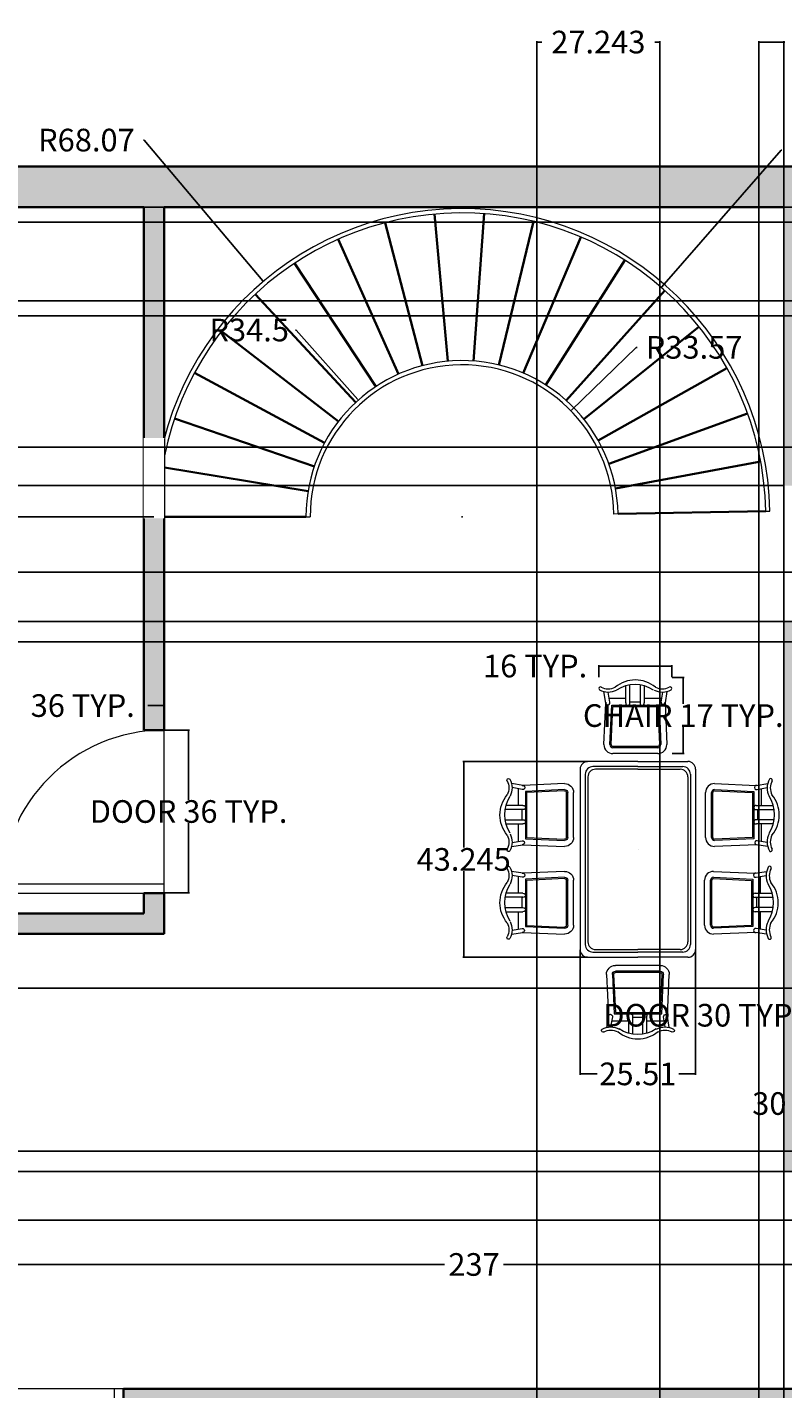
# Model space of a CAD drawing. Units: inches. Extents: x 2807 to 3326, y 2005 to 2580.
# Tile 10 of 12: x 2968 to 3135, y 2280 to 2580. Entities that reach past the tile are written whole.
import ezdxf

# ---------------------------------------------------------------- set-up
doc = ezdxf.new("R2010")
doc.units = ezdxf.units.IN
doc.header["$LTSCALE"] = 0.4
doc.set_wipeout_variables(frame=1)
for name, color, linetype, lineweight in [('A-ANNO-DIMS', 2, 'Continuous', 18), ('A-FLOR-STRS', 233, 'Continuous', 18), ('A-WALL-PATT', 231, 'Continuous', 13), ('DOORS', 144, 'Continuous', 18), ('Furniture', 7, 'Continuous', 15), ('WALL', 233, 'Continuous', 35)]:
    doc.layers.add(name, color=color, linetype=linetype, lineweight=lineweight)
doc.styles.get("Standard").update_dxf_attribs({"font": 'txt', "height": 5})
doc.dimstyles.get("Standard").update_dxf_attribs({"dimtxt": 0.18, "dimasz": 0.18, "dimexe": 0.18, "dimexo": 0.0625, "dimgap": 0.09, "dimtad": 0, "dimtih": 1, "dimtoh": 1, "dimdec": 4, "dimzin": 0, "dimdsep": 46, "dimtxsty": 'Standard', "dimcen": 0.09, "dimadec": 0, "dimazin": 0, "dimtfac": 1, "dimtdec": 4, "dimtofl": 0, "dimtmove": 0, "dimatfit": 3, "dimfxl": 1, "dimtolj": 1, "dimtzin": 0, "dimarcsym": 0})

# ---------------------------------------------------------------- blocks, each defined once
blk = doc.blocks.new('*U1')
at = {"layer": 'WALL'}
blk.add_line((0, -0.93), (0, -33.57), dxfattribs=at)
blk = doc.blocks.new('*U2')
at = {"layer": 'A-FLOR-STRS', "transparency": 16777216}
for p, rotation in [((3057.71, 2539.95), 5.233641268316883), ((3068.89, 2540.06), 355.8151569647967), ((3046.7, 2538.02), 14.65212557183719), ((3079.93, 2538.33), 346.3966726612762), ((3036.16, 2534.32), 24.07060987535752), ((3090.54, 2534.82), 336.9781883577561), ((3026.36, 2528.94), 33.48909417887789), ((3100.43, 2529.62), 327.5597040542357), ((3017.58, 2522.03), 42.90757848239826), ((3109.34, 2522.87), 318.1412197507153), ((3117.02, 2514.75), 308.7227354471949), ((3010.04, 2513.77), 52.32606278591863), ((3003.96, 2504.39), 61.74454708943897), ((3123.28, 2505.49), 299.3042511436746), ((2999.5, 2494.15), 71.16303139295928), ((3127.93, 2495.32), 289.8857668401543), ((3130.85, 2484.54), 280.4672825366339), ((2996.77, 2483.31), 80.58151569647963), ((2995.85, 2472.17), 90), ((3131.98, 2473.42), 271.0487982331135)]:
    blk.add_blockref('*U1', p, dxfattribs=dict(at, rotation=rotation))
blk = doc.blocks.new('DOOR-36')
for p, q in [((0, 0), (-36, 0)), ((-2, -35.94), (-2, 0)), ((0, -36), (0, 0))]:
    blk.add_line(p, q)
blk.add_arc((0, 0), 36, 180, 270)
blk = doc.blocks.new('CHAIR-DINING')
for p, q in [((-6.16, 6.94), (3.02, 6.53)), ((3.02, 6.53), (5.58, 6.94)), ((3.24, 5.62), (5.46, 6.04)), ((-8.14, -4.96), (-8.14, 4.96)), ((-6.84, -4.96), (-6.84, 4.96)), ((-6.56, -4.96), (-6.56, 4.96)), ((-6.16, 5.36), (2.25, 4.95)), ((-6.15, 5.64), (2.53, 5.22)), ((2.25, 4.95), (2.25, -5)), ((2.53, 5.22), (2.53, -5.28)), ((4.12, 5.78), (4.12, 2.1)), ((3.07, 2.1), (6.82, 2.1)), ((3.07, 1.2), (7.01, 1.2)), ((3.32, 1.2), (3.32, -1.08)), ((7.02, -1.08), (3.07, -1.08)), ((6.82, -1.98), (3.08, -1.98)), ((4.12, -1.98), (4.12, -5.82)), ((2.25, -5), (-6.16, -5.36)), ((2.53, -5.28), (-6.15, -5.64)), ((5.46, -6.04), (3.24, -5.67)), ((3.1, -6.58), (-6.16, -6.95)), ((5.58, -6.95), (3.1, -6.58))]:
    blk.add_line(p, q)
for centre, radius, start, end in [((-6.16, 4.96), 1.98, 90, 180), ((3.13, 6.07), 0.467, 76.2748, 283.7252), ((9.44, 5.97), 3.98, 151.1173, 207.5141), ((6.25, 7.7), 0.355, 326.5726, 147.7215), ((9.44, 5.97), 3.28, 150.9211, 207.5141), ((-6.16, 4.96), 0.68, 90, 180), ((-6.16, 4.96), 0.397, 90, 180), ((-0.48, 0.05), 7.58, 327.3186, 32.6814), ((1.16, 0), 6.98, 320.3459, 39.6541), ((2.98, 1.65), 0.463, 78.6748, 281.3252), ((2.98, -1.53), 0.463, 78.8014, 282.2085), ((-6.16, -4.96), 1.98, 180, 270), ((-6.16, -4.96), 0.68, 180, 270), ((-6.16, -4.96), 0.397, 180, 270), ((3.17, -6.13), 0.459, 80.8614, 279.1386), ((9.44, -5.97), 3.98, 152.4859, 208.8827), ((9.44, -5.97), 3.28, 152.4859, 208.022), ((6.25, -7.71), 0.355, 212.2785, 33.4274)]:
    blk.add_arc(centre, radius, start, end)
blk = doc.blocks.new('*D17')
at = {"layer": 'A-ANNO-DIMS', "color": 0, "lineweight": -2, "ltscale": 0.4, "transparency": 16777216}
for p, q in [((2998.13, 2425.08), (3003.65, 2425.08)), ((3003.47, 2424.9), (3003.47, 2409.67)), ((3003.47, 2389.26), (3003.47, 2404.49)), ((2998.13, 2389.08), (3003.65, 2389.08))]:
    blk.add_line(p, q, dxfattribs=at)
at = {"layer": 'A-ANNO-DIMS', "color": 0, "ltscale": 0.4, "transparency": 16777216}
for points in [[(3003.44, 2424.9), (3003.5, 2424.9), (3003.47, 2425.08)], [(3003.44, 2389.26), (3003.5, 2389.26), (3003.47, 2389.08)]]:
    blk.add_solid(points, dxfattribs=at)
at = {"layer": 'Defpoints', "color": 0, "ltscale": 0.4, "transparency": 16777216}
for p in [(2998.07, 2425.08), (2998.07, 2389.08), (3003.47, 2389.08)]:
    blk.add_point(p, dxfattribs=at)
at = {"layer": 'A-ANNO-DIMS', "color": 0, "ltscale": 0.4, "transparency": 16777216, "insert": (3003.47, 2407.08), "char_height": 5, "attachment_point": 5}
blk.add_mtext('\\A1;DOOR 36 TYP.', dxfattribs=at)
blk = doc.blocks.new('*D18')
at = {"layer": 'A-ANNO-DIMS', "color": 0, "lineweight": -2, "ltscale": 0.4, "transparency": 16777216}
for p, q in [((2962.07, 2425.14), (2962.07, 2430.66)), ((2962.25, 2430.48), (2965.69, 2430.48)), ((2997.89, 2430.48), (2994.44, 2430.48)), ((2998.07, 2425.14), (2998.07, 2430.66))]:
    blk.add_line(p, q, dxfattribs=at)
at = {"layer": 'A-ANNO-DIMS', "color": 0, "ltscale": 0.4, "transparency": 16777216}
for points in [[(2962.25, 2430.51), (2962.25, 2430.45), (2962.07, 2430.48)], [(2997.89, 2430.51), (2997.89, 2430.45), (2998.07, 2430.48)]]:
    blk.add_solid(points, dxfattribs=at)
at = {"layer": 'Defpoints', "color": 0, "ltscale": 0.4, "transparency": 16777216}
for p in [(2998.07, 2430.48), (2962.07, 2425.08), (2998.07, 2425.08)]:
    blk.add_point(p, dxfattribs=at)
at = {"layer": 'A-ANNO-DIMS', "color": 0, "ltscale": 0.4, "transparency": 16777216, "insert": (2980.07, 2430.48), "char_height": 5, "attachment_point": 5}
blk.add_mtext('\\A1;36 TYP.', dxfattribs=at)
blk = doc.blocks.new('*D19')
at = {"layer": 'A-ANNO-DIMS', "color": 0, "lineweight": -2, "ltscale": 0.4, "transparency": 16777216}
for p, q in [((3144.07, 2362.08), (3143.89, 2362.08)), ((3144.07, 2357.64), (3144.07, 2362.26)), ((3173.89, 2362.08), (3144.25, 2362.08)), ((3174.07, 2357.64), (3174.07, 2362.26))]:
    blk.add_line(p, q, dxfattribs=at)
at = {"layer": 'A-ANNO-DIMS', "color": 0, "ltscale": 0.4, "transparency": 16777216}
for points in [[(3144.25, 2362.11), (3144.25, 2362.05), (3144.07, 2362.08)], [(3173.89, 2362.11), (3173.89, 2362.05), (3174.07, 2362.08)]]:
    blk.add_solid(points, dxfattribs=at)
at = {"layer": 'Defpoints', "color": 0, "ltscale": 0.4, "transparency": 16777216}
for p in [(3144.07, 2362.08), (3144.07, 2357.58), (3174.07, 2357.58)]:
    blk.add_point(p, dxfattribs=at)
at = {"layer": 'A-ANNO-DIMS', "color": 0, "ltscale": 0.4, "transparency": 16777216, "insert": (3117.01, 2362.08), "char_height": 5, "attachment_point": 5}
blk.add_mtext('\\A1;DOOR 30 TYP.', dxfattribs=at)
blk = doc.blocks.new('*D20')
at = {"layer": 'A-ANNO-DIMS', "color": 0, "lineweight": -2, "ltscale": 0.4, "transparency": 16777216}
for p, q in [((3144, 2357.58), (3139.39, 2357.58)), ((3139.57, 2357.4), (3139.57, 2345.17)), ((3139.57, 2327.76), (3139.57, 2339.99)), ((3144, 2327.58), (3139.39, 2327.58))]:
    blk.add_line(p, q, dxfattribs=at)
at = {"layer": 'A-ANNO-DIMS', "color": 0, "ltscale": 0.4, "transparency": 16777216}
for points in [[(3139.54, 2357.4), (3139.6, 2357.4), (3139.57, 2357.58)], [(3139.54, 2327.76), (3139.6, 2327.76), (3139.57, 2327.58)]]:
    blk.add_solid(points, dxfattribs=at)
at = {"layer": 'Defpoints', "color": 0, "ltscale": 0.4, "transparency": 16777216}
for p in [(3144.07, 2357.58), (3139.57, 2327.58), (3144.07, 2327.58)]:
    blk.add_point(p, dxfattribs=at)
at = {"layer": 'A-ANNO-DIMS', "color": 0, "ltscale": 0.4, "transparency": 16777216, "insert": (3139.57, 2342.58), "char_height": 5, "attachment_point": 5}
blk.add_mtext('\\A1;30 TYP.', dxfattribs=at)
blk = doc.blocks.new('*D27')
at = {"layer": 'A-ANNO-DIMS', "color": 0, "lineweight": -2, "ltscale": 0.4, "transparency": 16777216}
for p, q in [((3110.36, 2436.69), (3113, 2436.69)), ((3112.82, 2436.51), (3112.82, 2430.86)), ((3112.82, 2420.04), (3112.82, 2425.68)), ((3110.36, 2419.86), (3113, 2419.86))]:
    blk.add_line(p, q, dxfattribs=at)
at = {"layer": 'A-ANNO-DIMS', "color": 0, "ltscale": 0.4, "transparency": 16777216}
for points in [[(3112.79, 2436.51), (3112.85, 2436.51), (3112.82, 2436.69)], [(3112.79, 2420.04), (3112.85, 2420.04), (3112.82, 2419.86)]]:
    blk.add_solid(points, dxfattribs=at)
at = {"layer": 'Defpoints', "color": 0, "ltscale": 0.4, "transparency": 16777216}
for p in [(3110.29, 2436.69), (3112.82, 2436.69), (3110.29, 2419.86)]:
    blk.add_point(p, dxfattribs=at)
at = {"layer": 'A-ANNO-DIMS', "color": 0, "ltscale": 0.4, "transparency": 16777216, "insert": (3112.82, 2428.27), "char_height": 5, "attachment_point": 5}
blk.add_mtext('\\A1;CHAIR 17 TYP.', dxfattribs=at)
blk = doc.blocks.new('*D28')
at = {"layer": 'A-ANNO-DIMS', "color": 0, "lineweight": -2, "ltscale": 0.4, "transparency": 16777216}
for p, q in [((3094.16, 2439.21), (3093.98, 2439.21)), ((3094.16, 2436.75), (3094.16, 2439.39)), ((3110.11, 2439.21), (3094.34, 2439.21)), ((3110.29, 2436.75), (3110.29, 2439.39))]:
    blk.add_line(p, q, dxfattribs=at)
at = {"layer": 'A-ANNO-DIMS', "color": 0, "ltscale": 0.4, "transparency": 16777216}
for points in [[(3094.34, 2439.24), (3094.34, 2439.18), (3094.16, 2439.21)], [(3110.11, 2439.24), (3110.11, 2439.18), (3110.29, 2439.21)]]:
    blk.add_solid(points, dxfattribs=at)
at = {"layer": 'Defpoints', "color": 0, "ltscale": 0.4, "transparency": 16777216}
for p in [(3094.16, 2439.21), (3094.16, 2436.69), (3110.29, 2436.69)]:
    blk.add_point(p, dxfattribs=at)
at = {"layer": 'A-ANNO-DIMS', "color": 0, "ltscale": 0.4, "transparency": 16777216, "insert": (3080.08, 2439.21), "char_height": 5, "attachment_point": 5}
blk.add_mtext('\\A1;16 TYP.', dxfattribs=at)
blk = doc.blocks.new('*D46')
at = {"layer": 'A-ANNO-DIMS', "color": 0, "lineweight": -2, "ltscale": 0.4, "transparency": 16777216}
for p, q in [((3279.5, 2327.58), (2816.94, 2327.58)), ((2817.12, 2327.4), (2817.12, 2324.79)), ((2817.12, 2317), (2817.12, 2319.61)), ((3279.5, 2316.82), (2816.94, 2316.82))]:
    blk.add_line(p, q, dxfattribs=at)
at = {"layer": 'A-ANNO-DIMS', "color": 0, "ltscale": 0.4, "transparency": 16777216}
for points in [[(2817.09, 2327.4), (2817.15, 2327.4), (2817.12, 2327.58)], [(2817.09, 2317), (2817.15, 2317), (2817.12, 2316.82)]]:
    blk.add_solid(points, dxfattribs=at)
at = {"layer": 'Defpoints', "color": 0, "ltscale": 0.4, "transparency": 16777216}
for p in [(2817.12, 2327.58), (3279.57, 2327.58), (3279.57, 2316.82)]:
    blk.add_point(p, dxfattribs=at)
at = {"layer": 'A-ANNO-DIMS', "color": 0, "ltscale": 0.4, "transparency": 16777216, "insert": (2817.12, 2322.2), "char_height": 5, "attachment_point": 5}
blk.add_mtext('\\A1;10.754', dxfattribs=at)
blk = doc.blocks.new('*D47')
at = {"layer": 'A-ANNO-DIMS', "color": 0, "lineweight": -2, "ltscale": 0.4, "transparency": 16777216}
for p, q in [((3279.504691, 2368.076496), (2816.937191, 2368.076496)), ((2817.117191, 2367.896496), (2817.117191, 2352.666496)), ((2817.117191, 2332.256496), (2817.117191, 2347.486496)), ((3279.504691, 2332.076496), (2816.937191, 2332.076496))]:
    blk.add_line(p, q, dxfattribs=at)
at = {"layer": 'A-ANNO-DIMS', "color": 0, "ltscale": 0.4, "transparency": 16777216}
for points in [[(2817.087191, 2367.896496), (2817.147191, 2367.896496), (2817.117191, 2368.076496)], [(2817.087191, 2332.256496), (2817.147191, 2332.256496), (2817.117191, 2332.076496)]]:
    blk.add_solid(points, dxfattribs=at)
at = {"layer": 'Defpoints', "color": 0, "ltscale": 0.4, "transparency": 16777216}
for p in [(2817.117191, 2368.076496), (3279.567191, 2368.076496), (3279.567191, 2332.076496)]:
    blk.add_point(p, dxfattribs=at)
at = {"layer": 'A-ANNO-DIMS', "color": 0, "ltscale": 0.4, "transparency": 16777216, "insert": (2817.117191, 2350.076496), "char_height": 5, "attachment_point": 5}
blk.add_mtext('\\A1;36', dxfattribs=at)
blk = doc.blocks.new('*D50')
at = {"layer": 'A-ANNO-DIMS', "color": 0, "lineweight": -2, "ltscale": 0.4, "transparency": 16777216}
for p, q in [((3139.504691, 2540.576496), (2816.937191, 2540.576496)), ((2817.117191, 2540.396496), (2817.117191, 2531.166496)), ((2817.117191, 2516.756496), (2817.117191, 2525.986496)), ((3139.504691, 2516.576496), (2816.937191, 2516.576496))]:
    blk.add_line(p, q, dxfattribs=at)
at = {"layer": 'A-ANNO-DIMS', "color": 0, "ltscale": 0.4, "transparency": 16777216}
for points in [[(2817.087191, 2540.396496), (2817.147191, 2540.396496), (2817.117191, 2540.576496)], [(2817.087191, 2516.756496), (2817.147191, 2516.756496), (2817.117191, 2516.576496)]]:
    blk.add_solid(points, dxfattribs=at)
at = {"layer": 'Defpoints', "color": 0, "ltscale": 0.4, "transparency": 16777216}
for p in [(2817.117191, 2540.576496), (3139.567191, 2540.576496), (3139.567191, 2516.576496)]:
    blk.add_point(p, dxfattribs=at)
at = {"layer": 'A-ANNO-DIMS', "color": 0, "ltscale": 0.4, "transparency": 16777216, "insert": (2817.117191, 2528.576496), "char_height": 5, "attachment_point": 5}
blk.add_mtext('\\A1;24', dxfattribs=at)
blk = doc.blocks.new('*D51')
at = {"layer": 'A-ANNO-DIMS', "color": 0, "lineweight": -2, "ltscale": 0.4, "transparency": 16777216}
for p, q in [((3135.004691, 2479.076496), (2816.937191, 2479.076496)), ((2817.117191, 2478.896496), (2817.117191, 2466.666496)), ((2817.117191, 2449.256496), (2817.117191, 2461.486496)), ((3135.004691, 2449.076496), (2816.937191, 2449.076496))]:
    blk.add_line(p, q, dxfattribs=at)
at = {"layer": 'A-ANNO-DIMS', "color": 0, "ltscale": 0.4, "transparency": 16777216}
for points in [[(2817.087191, 2478.896496), (2817.147191, 2478.896496), (2817.117191, 2479.076496)], [(2817.087191, 2449.256496), (2817.147191, 2449.256496), (2817.117191, 2449.076496)]]:
    blk.add_solid(points, dxfattribs=at)
at = {"layer": 'Defpoints', "color": 0, "ltscale": 0.4, "transparency": 16777216}
for p in [(2817.117191, 2479.076496), (3135.067191, 2479.076496), (3135.067191, 2449.076496)]:
    blk.add_point(p, dxfattribs=at)
at = {"layer": 'A-ANNO-DIMS', "color": 0, "ltscale": 0.4, "transparency": 16777216, "insert": (2817.117191, 2464.076496), "char_height": 5, "attachment_point": 5}
blk.add_mtext('\\A1;30', dxfattribs=at)
blk = doc.blocks.new('*D52')
at = {"layer": 'A-ANNO-DIMS', "color": 0, "lineweight": -2, "ltscale": 0.4, "transparency": 16777216}
for p, q in [((2941.5, 2540.58), (2816.94, 2540.58)), ((2817.12, 2540.4), (2817.12, 2508.96)), ((2817.12, 2472.35), (2817.12, 2503.78)), ((2995.79, 2472.17), (2816.94, 2472.17))]:
    blk.add_line(p, q, dxfattribs=at)
at = {"layer": 'A-ANNO-DIMS', "color": 0, "ltscale": 0.4, "transparency": 16777216}
for points in [[(2817.09, 2540.4), (2817.15, 2540.4), (2817.12, 2540.58)], [(2817.09, 2472.35), (2817.15, 2472.35), (2817.12, 2472.17)]]:
    blk.add_solid(points, dxfattribs=at)
at = {"layer": 'Defpoints', "color": 0, "ltscale": 0.4, "transparency": 16777216}
for p in [(2941.57, 2540.58), (2817.12, 2472.17), (2995.85, 2472.17)]:
    blk.add_point(p, dxfattribs=at)
at = {"layer": 'A-ANNO-DIMS', "color": 0, "ltscale": 0.4, "transparency": 16777216, "insert": (2817.12, 2506.37), "char_height": 5, "attachment_point": 5}
blk.add_mtext('\\A1;68.4', dxfattribs=at)
blk = doc.blocks.new('*D54')
at = {"layer": 'A-ANNO-DIMS', "color": 0, "lineweight": -2, "ltscale": 0.4, "transparency": 16777216}
for p, q in [((3198.393277, 2537.214927), (2816.937191, 2537.214927)), ((2817.117191, 2537.034927), (2817.117191, 2531.143527)), ((2817.117191, 2520.072127), (2817.117191, 2525.963527)), ((3198.393277, 2519.892127), (2816.937191, 2519.892127))]:
    blk.add_line(p, q, dxfattribs=at)
at = {"layer": 'A-ANNO-DIMS', "color": 0, "ltscale": 0.4, "transparency": 16777216}
for points in [[(2817.087191, 2537.034927), (2817.147191, 2537.034927), (2817.117191, 2537.214927)], [(2817.087191, 2520.072127), (2817.147191, 2520.072127), (2817.117191, 2519.892127)]]:
    blk.add_solid(points, dxfattribs=at)
at = {"layer": 'Defpoints', "color": 0, "ltscale": 0.4, "transparency": 16777216}
for p in [(2817.117191, 2537.214927), (3198.455777, 2537.214927), (3198.455777, 2519.892127)]:
    blk.add_point(p, dxfattribs=at)
at = {"layer": 'A-ANNO-DIMS', "color": 0, "ltscale": 0.4, "transparency": 16777216, "insert": (2817.117191, 2528.553527), "char_height": 5, "attachment_point": 5}
blk.add_mtext('\\A1;17.323', dxfattribs=at)
blk = doc.blocks.new('*D56')
at = {"layer": 'A-ANNO-DIMS', "color": 0, "lineweight": -2, "ltscale": 0.4, "transparency": 16777216}
for p, q in [((3258.250937, 2487.533633), (2816.937191, 2487.533633)), ((2817.117191, 2487.353633), (2817.117191, 2476.344133)), ((2817.117191, 2460.154633), (2817.117191, 2471.164133)), ((3258.250937, 2459.974633), (2816.937191, 2459.974633))]:
    blk.add_line(p, q, dxfattribs=at)
at = {"layer": 'A-ANNO-DIMS', "color": 0, "ltscale": 0.4, "transparency": 16777216}
for points in [[(2817.087191, 2487.353633), (2817.147191, 2487.353633), (2817.117191, 2487.533633)], [(2817.087191, 2460.154633), (2817.147191, 2460.154633), (2817.117191, 2459.974633)]]:
    blk.add_solid(points, dxfattribs=at)
at = {"layer": 'Defpoints', "color": 0, "ltscale": 0.4, "transparency": 16777216}
for p in [(2817.117191, 2487.533633), (3258.313437, 2487.533633), (3258.313437, 2459.974633)]:
    blk.add_point(p, dxfattribs=at)
at = {"layer": 'A-ANNO-DIMS', "color": 0, "ltscale": 0.4, "transparency": 16777216, "insert": (2817.117191, 2473.754133), "char_height": 5, "attachment_point": 5}
blk.add_mtext('\\A1;27.56', dxfattribs=at)
blk = doc.blocks.new('*D59')
at = {"layer": 'A-ANNO-DIMS', "color": 0, "lineweight": -2, "ltscale": 0.4, "transparency": 16777216}
for p, q in [((3091.672098, 2418.126241), (3064.104598, 2418.126241)), ((3064.284598, 2417.946241), (3064.284598, 2399.093945)), ((3064.284598, 2375.061649), (3064.284598, 2393.913945)), ((3091.672098, 2374.881649), (3064.104598, 2374.881649))]:
    blk.add_line(p, q, dxfattribs=at)
at = {"layer": 'A-ANNO-DIMS', "color": 0, "ltscale": 0.4, "transparency": 16777216}
for points in [[(3064.254598, 2417.946241), (3064.314598, 2417.946241), (3064.284598, 2418.126241)], [(3064.254598, 2375.061649), (3064.314598, 2375.061649), (3064.284598, 2374.881649)]]:
    blk.add_solid(points, dxfattribs=at)
at = {"layer": 'Defpoints', "color": 0, "ltscale": 0.4, "transparency": 16777216}
for p in [(3064.284598, 2418.126241), (3091.734598, 2418.126241), (3091.734598, 2374.881649)]:
    blk.add_point(p, dxfattribs=at)
at = {"layer": 'A-ANNO-DIMS', "color": 0, "ltscale": 0.4, "transparency": 16777216, "insert": (3064.284598, 2396.503945), "char_height": 5, "attachment_point": 5}
blk.add_mtext('\\A1;43.245', dxfattribs=at)
blk = doc.blocks.new('*D60')
at = {"layer": 'A-ANNO-DIMS', "color": 0, "lineweight": -2, "ltscale": 0.4, "transparency": 16777216}
for p, q in [((3090.03, 2376.52), (3090.03, 2348.95)), ((3115.55, 2376.52), (3115.55, 2348.95)), ((3090.21, 2349.13), (3093.77, 2349.13)), ((3115.37, 2349.13), (3111.81, 2349.13))]:
    blk.add_line(p, q, dxfattribs=at)
at = {"layer": 'A-ANNO-DIMS', "color": 0, "ltscale": 0.4, "transparency": 16777216}
for points in [[(3090.21, 2349.16), (3090.21, 2349.1), (3090.03, 2349.13)], [(3115.37, 2349.16), (3115.37, 2349.1), (3115.55, 2349.13)]]:
    blk.add_solid(points, dxfattribs=at)
at = {"layer": 'Defpoints', "color": 0, "ltscale": 0.4, "transparency": 16777216}
for p in [(3090.03, 2376.58), (3115.55, 2376.58), (3090.03, 2349.13)]:
    blk.add_point(p, dxfattribs=at)
at = {"layer": 'A-ANNO-DIMS', "color": 0, "ltscale": 0.4, "transparency": 16777216, "insert": (3102.79, 2349.13), "char_height": 5, "attachment_point": 5}
blk.add_mtext('\\A1;25.51', dxfattribs=at)
blk = doc.blocks.new('*D64')
at = {"layer": 'A-ANNO-DIMS', "color": 0, "lineweight": -2, "ltscale": 0.4, "transparency": 16777216}
for p, q in [((3080.43, 2237.61), (3080.43, 2577.21)), ((3080.61, 2577.03), (3081.58, 2577.03)), ((3107.49, 2577.03), (3106.52, 2577.03)), ((3107.67, 2237.61), (3107.67, 2577.21))]:
    blk.add_line(p, q, dxfattribs=at)
at = {"layer": 'A-ANNO-DIMS', "color": 0, "ltscale": 0.4, "transparency": 16777216}
for points in [[(3080.61, 2577.06), (3080.61, 2577), (3080.43, 2577.03)], [(3107.49, 2577.06), (3107.49, 2577), (3107.67, 2577.03)]]:
    blk.add_solid(points, dxfattribs=at)
at = {"layer": 'Defpoints', "color": 0, "ltscale": 0.4, "transparency": 16777216}
for p in [(3107.67, 2577.03), (3080.43, 2237.55), (3107.67, 2237.55)]:
    blk.add_point(p, dxfattribs=at)
at = {"layer": 'A-ANNO-DIMS', "color": 0, "ltscale": 0.4, "transparency": 16777216, "insert": (3094.05, 2577.03), "char_height": 5, "attachment_point": 5}
blk.add_mtext('\\A1;27.243', dxfattribs=at)
blk = doc.blocks.new('*D66')
at = {"layer": 'A-ANNO-DIMS', "color": 0, "lineweight": -2, "ltscale": 0.4, "transparency": 16777216}
for p, q in [((3129.534988, 2263.581941), (3129.534988, 2577.206496)), ((3129.714988, 2577.026496), (3134.887191, 2577.026496)), ((3135.067191, 2275.138996), (3135.067191, 2577.206496)), ((3135.067191, 2577.026496), (3135.247191, 2577.026496))]:
    blk.add_line(p, q, dxfattribs=at)
at = {"layer": 'A-ANNO-DIMS', "color": 0, "ltscale": 0.4, "transparency": 16777216}
for points in [[(3129.714988, 2577.056496), (3129.714988, 2576.996496), (3129.534988, 2577.026496)], [(3134.887191, 2577.056496), (3134.887191, 2576.996496), (3135.067191, 2577.026496)]]:
    blk.add_solid(points, dxfattribs=at)
at = {"layer": 'Defpoints', "color": 0, "ltscale": 0.4, "transparency": 16777216}
for p in [(3135.067191, 2577.026496), (3135.067191, 2275.076496), (3129.534988, 2263.519441)]:
    blk.add_point(p, dxfattribs=at)
at = {"layer": 'A-ANNO-DIMS', "color": 0, "ltscale": 0.4, "transparency": 16777216, "insert": (3145.337191, 2577.026496), "char_height": 5, "attachment_point": 5}
blk.add_mtext('\\A1;5.532', dxfattribs=at)
blk = doc.blocks.new('*D71')
at = {"layer": 'A-ANNO-DIMS', "color": 0, "lineweight": -2, "ltscale": 0.4, "transparency": 16777216}
for p, q in [((3139.5, 2449.08), (2816.94, 2449.08)), ((2817.12, 2449.08), (2817.12, 2449.26)), ((2817.12, 2449.26), (2817.3, 2449.26)), ((2817.12, 2444.76), (2817.12, 2448.9)), ((3139.5, 2444.58), (2816.94, 2444.58))]:
    blk.add_line(p, q, dxfattribs=at)
at = {"layer": 'A-ANNO-DIMS', "color": 0, "ltscale": 0.4, "transparency": 16777216}
for points in [[(2817.09, 2448.9), (2817.15, 2448.9), (2817.12, 2449.08)], [(2817.09, 2444.76), (2817.15, 2444.76), (2817.12, 2444.58)]]:
    blk.add_solid(points, dxfattribs=at)
at = {"layer": 'Defpoints', "color": 0, "ltscale": 0.4, "transparency": 16777216}
for p in [(2817.12, 2449.08), (3139.57, 2449.08), (3139.57, 2444.58)]:
    blk.add_point(p, dxfattribs=at)
at = {"layer": 'A-ANNO-DIMS', "color": 0, "ltscale": 0.4, "transparency": 16777216, "insert": (2822.63, 2449.26), "char_height": 5, "attachment_point": 5}
blk.add_mtext('\\A1;4.5', dxfattribs=at)
blk = doc.blocks.new('*D72')
at = {"layer": 'A-ANNO-DIMS', "color": 0, "lineweight": -2, "ltscale": 0.4, "transparency": 16777216}
for p, q in [((2948.07, 2279.64), (2948.07, 2307.21)), ((2948.25, 2307.03), (3060.05, 2307.03)), ((3184.89, 2307.03), (3073.09, 2307.03)), ((3185.07, 2279.64), (3185.07, 2307.21))]:
    blk.add_line(p, q, dxfattribs=at)
at = {"layer": 'A-ANNO-DIMS', "color": 0, "ltscale": 0.4, "transparency": 16777216}
for points in [[(2948.25, 2307.06), (2948.25, 2307), (2948.07, 2307.03)], [(3184.89, 2307.06), (3184.89, 2307), (3185.07, 2307.03)]]:
    blk.add_solid(points, dxfattribs=at)
at = {"layer": 'Defpoints', "color": 0, "ltscale": 0.4, "transparency": 16777216}
for p in [(3185.07, 2307.03), (2948.07, 2279.58), (3185.07, 2279.58)]:
    blk.add_point(p, dxfattribs=at)
at = {"layer": 'A-ANNO-DIMS', "color": 0, "ltscale": 0.4, "transparency": 16777216, "insert": (3066.57, 2307.03), "char_height": 5, "attachment_point": 5}
blk.add_mtext('\\A1;237', dxfattribs=at)
blk = doc.blocks.new('*D74')
at = {"layer": 'A-ANNO-DIMS', "color": 0, "lineweight": -2, "ltscale": 0.4, "transparency": 16777216}
for p, q in [((2993.47, 2555.38), (2993.65, 2555.38)), ((2993.65, 2555.38), (3019.89, 2524.31)), ((3063.83, 2472.17), (3064.01, 2472.17)), ((3063.92, 2472.08), (3063.92, 2472.26))]:
    blk.add_line(p, q, dxfattribs=at)
at = {"layer": 'A-ANNO-DIMS', "color": 0, "ltscale": 0.4, "transparency": 16777216}
blk.add_solid([(3019.91, 2524.33), (3019.86, 2524.29), (3020, 2524.18)], dxfattribs=at)
at = {"layer": 'Defpoints', "color": 0, "ltscale": 0.4, "transparency": 16777216}
for p in [(3020, 2524.18), (3063.92, 2472.17)]:
    blk.add_point(p, dxfattribs=at)
at = {"layer": 'A-ANNO-DIMS', "color": 0, "ltscale": 0.4, "transparency": 16777216, "insert": (2980.88, 2555.38), "char_height": 5, "attachment_point": 5}
blk.add_mtext('\\A1;R68.07', dxfattribs=at)
blk = doc.blocks.new('*D75')
at = {"layer": 'A-ANNO-DIMS', "color": 0, "lineweight": -2, "ltscale": 0.4, "transparency": 16777216}
for p, q in [((3134.45, 2553.19), (3108.12, 2522.94)), ((3134.63, 2553.19), (3134.45, 2553.19)), ((3063.83, 2472.17), (3064.01, 2472.17)), ((3063.92, 2472.08), (3063.92, 2472.26))]:
    blk.add_line(p, q, dxfattribs=at)
at = {"layer": 'A-ANNO-DIMS', "color": 0, "ltscale": 0.4, "transparency": 16777216}
blk.add_solid([(3108.09, 2522.96), (3108.14, 2522.92), (3108, 2522.81)], dxfattribs=at)
at = {"layer": 'Defpoints', "color": 0, "ltscale": 0.4, "transparency": 16777216}
for p in [(3108, 2522.81), (3063.92, 2472.17)]:
    blk.add_point(p, dxfattribs=at)
at = {"layer": 'A-ANNO-DIMS', "color": 0, "ltscale": 0.4, "transparency": 16777216, "insert": (3146.86, 2553.19), "char_height": 5, "attachment_point": 5}
blk.add_mtext('\\A1;R67.14', dxfattribs=at)
blk = doc.blocks.new('*D76')
at = {"layer": 'A-ANNO-DIMS', "color": 0, "lineweight": -2, "ltscale": 0.4, "transparency": 16777216}
for p, q in [((3027.07, 2513.43), (3027.25, 2513.43)), ((3027.25, 2513.43), (3040.88, 2498.09)), ((3063.83, 2472.17), (3064.01, 2472.17)), ((3063.92, 2472.08), (3063.92, 2472.26))]:
    blk.add_line(p, q, dxfattribs=at)
at = {"layer": 'A-ANNO-DIMS', "color": 0, "ltscale": 0.4, "transparency": 16777216}
blk.add_solid([(3040.9, 2498.11), (3040.86, 2498.07), (3041, 2497.96)], dxfattribs=at)
at = {"layer": 'Defpoints', "color": 0, "ltscale": 0.4, "transparency": 16777216}
for p in [(3041, 2497.96), (3063.92, 2472.17)]:
    blk.add_point(p, dxfattribs=at)
at = {"layer": 'A-ANNO-DIMS', "color": 0, "ltscale": 0.4, "transparency": 16777216, "insert": (3016.86, 2513.43), "char_height": 5, "attachment_point": 5}
blk.add_mtext('\\A1;R34.5', dxfattribs=at)
blk = doc.blocks.new('*D77')
at = {"layer": 'A-ANNO-DIMS', "color": 0, "lineweight": -2, "ltscale": 0.4, "transparency": 16777216}
for p, q in [((3102.44, 2509.6), (3088.12, 2495.69)), ((3102.62, 2509.6), (3102.44, 2509.6)), ((3063.83, 2472.17), (3064.01, 2472.17)), ((3063.92, 2472.08), (3063.92, 2472.26))]:
    blk.add_line(p, q, dxfattribs=at)
at = {"layer": 'A-ANNO-DIMS', "color": 0, "ltscale": 0.4, "transparency": 16777216}
blk.add_solid([(3088.1, 2495.71), (3088.14, 2495.67), (3087.99, 2495.56)], dxfattribs=at)
at = {"layer": 'Defpoints', "color": 0, "ltscale": 0.4, "transparency": 16777216}
for p in [(3087.99, 2495.56), (3063.92, 2472.17)]:
    blk.add_point(p, dxfattribs=at)
at = {"layer": 'A-ANNO-DIMS', "color": 0, "ltscale": 0.4, "transparency": 16777216, "insert": (3115.21, 2509.6), "char_height": 5, "attachment_point": 5}
blk.add_mtext('\\A1;R33.57', dxfattribs=at)

msp = doc.modelspace()

# ---------------------------------------------------------------- hatches: boundary and pattern name
at = {"layer": 'A-WALL-PATT', "ltscale": 0.4}
h = msp.add_hatch(color=256, dxfattribs=at)
h.dxf.hatch_style = 1
h.paths.add_polyline_path([(3288.5672, 2549.5765), (2941.5672, 2549.5765), (2941.5672, 2540.5765), (2993.5672, 2540.5765), (2993.5672, 2489.5693), (2998.0672, 2489.5693), (2998.0672, 2540.5765), (3135.0672, 2540.5765), (3135.0672, 2479.0765), (3139.5672, 2479.0765), (3139.5672, 2540.5765), (3279.5672, 2540.5765), (3279.5672, 2510.5765), (3288.5672, 2510.5765)])
h.paths.add_polyline_path([(2905.5672, 2549.5765), (2844.5672, 2549.5765), (2844.5672, 2445.94), (2853.5672, 2445.94), (2853.5672, 2540.5765), (2905.5672, 2540.5765)])
h.paths.add_polyline_path([(2853.5672, 2409.94), (2844.5672, 2409.94), (2844.5672, 2371.3497), (2853.5672, 2371.3497), (2853.5672, 2380.0765), (2909.0672, 2380.0765), (2909.0672, 2384.5765), (2853.5672, 2384.5765)])
h.paths.add_polyline_path([(2998.0672, 2389.0765), (2993.5672, 2389.0765), (2993.5672, 2384.5765), (2939.0672, 2384.5765), (2939.0672, 2380.0765), (2943.5672, 2380.0765), (2943.5672, 2314.0765), (2948.0672, 2314.0765), (2948.0672, 2380.0765), (2998.0672, 2380.0765)])
h.paths.add_polyline_path([(2998.0672, 2471.8029), (2993.5672, 2471.8029), (2993.5672, 2425.0765), (2998.0672, 2425.0765)])
h.paths.add_polyline_path([(2953.0672, 2279.5765), (2948.0672, 2279.5765), (2948.0672, 2284.0765), (2943.5672, 2284.0765), (2943.5672, 2279.5765), (2853.5672, 2279.5765), (2853.5672, 2289.0663), (2844.5672, 2289.0663), (2844.5672, 2227.8961), (2853.5672, 2227.8961), (2853.5672, 2275.0765), (2953.0672, 2275.0765)])
h.paths.add_polyline_path([(2943.5672, 2332.0765), (2853.5672, 2332.0765), (2853.5672, 2347.3497), (2844.5672, 2347.3497), (2844.5672, 2313.0663), (2853.5672, 2313.0663), (2853.5672, 2327.5765), (2943.5672, 2327.5765)])
h.paths.add_polyline_path([(3144.0672, 2279.5765), (2993.5672, 2279.5765), (2989.0672, 2279.5765), (2989.0672, 2275.0765), (2993.5672, 2275.0765), (2993.5672, 2144.5765), (2984.5672, 2144.5765), (2984.5672, 2135.5765), (2993.5672, 2135.5765), (2993.5672, 2120.0765), (3036.5672, 2120.0765), (3036.5672, 2129.0765), (2998.0672, 2129.0765), (2998.0672, 2275.0765), (3135.0672, 2275.0765), (3135.0672, 2129.0765), (3096.5672, 2129.0765), (3096.5672, 2120.0765), (3139.5672, 2120.0765), (3139.5672, 2135.5765), (3148.5672, 2135.5765), (3148.5672, 2144.5765), (3139.5672, 2144.5765), (3139.5672, 2275.0765), (3144.0672, 2275.0765)])
h.paths.add_polyline_path([(2984.5672, 2144.5765), (2925.9914, 2144.5765), (2925.9914, 2135.5765), (2984.5672, 2135.5765)])
h.paths.add_polyline_path([(2889.9914, 2144.5765), (2853.5672, 2144.5765), (2853.5672, 2191.8961), (2844.5672, 2191.8961), (2844.5672, 2135.5765), (2889.9914, 2135.5765)])
h.paths.add_polyline_path([(3196.0672, 2144.5765), (3148.5672, 2144.5765), (3148.5672, 2135.5765), (3196.0672, 2135.5765)])
h.paths.add_polyline_path([(3288.5672, 2191.8265), (3279.5672, 2191.8265), (3279.5672, 2144.5765), (3232.0672, 2144.5765), (3232.0672, 2135.5765), (3288.5672, 2135.5765)])
h.paths.add_polyline_path([(3288.5672, 2292.8229), (3279.5672, 2292.8229), (3279.5672, 2291.4371), (3279.5672, 2279.5765), (3189.5672, 2279.5765), (3189.5672, 2293.0765), (3185.0672, 2293.0765), (3185.0672, 2279.5765), (3180.0672, 2279.5765), (3180.0672, 2275.0765), (3279.5672, 2275.0765), (3279.5672, 2227.8265), (3288.5672, 2227.8265)])
h.paths.add_polyline_path([(3288.5672, 2368.0765), (3279.5672, 2368.0765), (3279.5672, 2332.0765), (3174.0672, 2332.0765), (3174.0672, 2327.5765), (3185.0672, 2327.5765), (3189.5672, 2327.5765), (3279.5672, 2327.5765), (3279.5672, 2316.8229), (3288.5672, 2316.8229)])
h.paths.add_polyline_path([(3288.5672, 2474.5765), (3279.5672, 2474.5765), (3279.5672, 2444.5765), (3139.5672, 2444.5765), (3139.5672, 2449.0765), (3135.0672, 2449.0765), (3135.0672, 2327.5765), (3144.0672, 2327.5765), (3144.0672, 2332.0765), (3139.5672, 2332.0765), (3139.5672, 2440.0765), (3279.5672, 2440.0765), (3279.5672, 2404.0765), (3288.5672, 2404.0765)])

# ---------------------------------------------------------------- linework, layer by layer
at = {"layer": 'A-FLOR-STRS'}
for p, q in [((2996.7824, 2472.1697), (2995.85, 2472.1697)), ((3029.4181, 2472.1697), (3030.3506, 2472.1697)), ((3098.4192, 2472.8013), (3097.4811, 2472.7841)), ((3131.0436, 2473.3986), (3131.9759, 2473.4156))]:
    msp.add_line(p, q, dxfattribs=at)
for radius in [68.0687, 67.1362, 34.5006, 33.5681]:
    msp.add_arc((3063.9187, 2472.1697), radius, 1.048798, 180, dxfattribs=at)
at = {"layer": 'Furniture'}
for p, q in [((3102.7897, 2418.1262), (3091.7346, 2418.1262)), ((3102.7897, 2418.1262), (3113.8448, 2418.1262)), ((3090.0338, 2416.4255), (3090.0338, 2396.5039)), ((3091.1677, 2415.2916), (3091.1677, 2396.5039)), ((3102.7897, 2416.9924), (3092.8685, 2416.9924)), ((3102.7897, 2416.4255), (3093.4354, 2416.4255)), ((3102.7897, 2416.9924), (3112.7109, 2416.9924)), ((3102.7897, 2416.4255), (3112.144, 2416.4255)), ((3114.4117, 2415.2916), (3114.4117, 2396.5039)), ((3115.5456, 2416.4255), (3115.5456, 2396.5039)), ((3091.7346, 2414.7247), (3091.7346, 2396.5039)), ((3113.8448, 2414.7247), (3113.8448, 2396.5039)), ((3090.0338, 2396.5039), (3090.0338, 2376.5824)), ((3091.1677, 2396.5039), (3091.1677, 2377.7163)), ((3091.7346, 2396.5039), (3091.7346, 2378.2832)), ((3113.8448, 2396.5039), (3113.8448, 2378.2832)), ((3114.4117, 2396.5039), (3114.4117, 2377.7163)), ((3115.5456, 2396.5039), (3115.5456, 2376.5824)), ((3092.8685, 2376.0155), (3102.7897, 2376.0155)), ((3093.4354, 2376.5824), (3102.7897, 2376.5824)), ((3112.144, 2376.5824), (3102.7897, 2376.5824)), ((3112.7109, 2376.0155), (3102.7897, 2376.0155)), ((3091.7346, 2374.8816), (3102.7897, 2374.8816)), ((3113.8448, 2374.8816), (3102.7897, 2374.8816))]:
    msp.add_line(p, q, dxfattribs=at)
for centre, start, end in [((3091.7346, 2416.4255), 90, 180), ((3113.8448, 2416.4255), 0, 90), ((3092.8685, 2415.2916), 90, 180), ((3093.4354, 2414.7247), 90, 180), ((3112.144, 2414.7247), 0, 90), ((3112.7109, 2415.2916), 0, 90), ((3091.7346, 2376.5824), 180, 270), ((3092.8685, 2377.7163), 180, 270), ((3093.4354, 2378.2832), 180, 270), ((3112.144, 2378.2832), 270, 0), ((3112.7109, 2377.7163), 270, 0), ((3113.8448, 2376.5824), 270, 0)]:
    msp.add_arc(centre, 1.7008, start, end, dxfattribs=at)
at = {"layer": 'WALL'}
for p, q in [((2844.5672, 2549.5765), (3288.5672, 2549.5765)), ((2853.5672, 2540.5765), (2993.5672, 2540.5765)), ((2993.5672, 2540.5765), (2993.5672, 2425.0765)), ((2998.0672, 2540.5765), (3135.0672, 2540.5765)), ((2998.0672, 2425.0765), (2998.0672, 2540.5765)), ((2993.5672, 2425.0765), (2998.0672, 2425.0765)), ((2993.5672, 2384.5765), (2993.5672, 2389.0765)), ((2993.5672, 2389.0765), (2998.0672, 2389.0765)), ((2998.0672, 2380.0765), (2998.0672, 2389.0765)), ((2939.0672, 2384.5765), (2993.5672, 2384.5765)), ((2948.0672, 2380.0765), (2998.0672, 2380.0765)), ((2989.0672, 2275.0765), (2989.0672, 2279.5765)), ((2989.0672, 2279.5765), (2993.5672, 2279.5765)), ((2993.5672, 2279.5765), (3144.0672, 2279.5765))]:
    msp.add_line(p, q, dxfattribs=at)

# ---------------------------------------------------------------- block references
at = {"layer": 'A-FLOR-STRS'}
msp.add_blockref('*U2', (0, 0), dxfattribs=at)
at = {"layer": 'DOORS', "rotation": 269.9999999999992}
msp.add_blockref('DOOR-36', (2998.0672, 2389.0765), dxfattribs=at)
at = {"layer": 'DOORS'}
msp.add_blockref('DOOR-36', (2989.0672, 2279.5765), dxfattribs=at)
at = {"layer": 'Furniture', "rotation": 89.9999999999846}
msp.add_blockref('CHAIR-DINING', (3102.2274, 2428.0056), dxfattribs=at)
at = {"layer": 'Furniture', "extrusion": (0, 0, -1), "zscale": -1}
for p in [(-3080.4427, 2406.307), (-3080.4427, 2386.9241)]:
    msp.add_blockref('CHAIR-DINING', p, dxfattribs=at)
at = {"layer": 'Furniture'}
for p in [(3125.901, 2406.307), (3125.6728, 2386.9241)]:
    msp.add_blockref('CHAIR-DINING', p, dxfattribs=at)
at = {"layer": 'Furniture', "extrusion": (0, 0, -1), "zscale": -1, "rotation": 269.9999999999597}
msp.add_blockref('CHAIR-DINING', (-3102.7895, 2364.9451), dxfattribs=at)

# ---------------------------------------------------------------- texts
at = {"layer": 'Furniture', "flags": 9}
for tag, s in [('ZSIZE', '0.0429'), ('XSIZE', '1591.9460'), ('YSIZE', '2019.3631')]:
    msp.add_attdef(tag, (3103.0363, 2398.7729), s, height=0.01969, rotation=180, dxfattribs=at)

# ---------------------------------------------------------------- dimensions: what is measured, and where the dimension line sits
at = {"layer": 'A-ANNO-DIMS', "ltscale": 0.4}
for base, p1, p2, picture, middle in [((3107.6694, 2577.0265), (3080.4262, 2237.5518), (3107.6694, 2237.5518), '*D64', (3094.0478, 2577.0265)), ((3135.0672, 2577.0265), (3129.535, 2263.5194), (3135.0672, 2275.0765), '*D66', (3145.3372, 2577.0265))]:
    dim = msp.add_linear_dim(base=base, p1=p1, p2=p2, dimstyle='Standard', override={"dimdec": 3, "dimlfac": 1, "dimrnd": 0, "dimzin": 0, "dimdsep": 46, "dimlunit": 2}, dxfattribs=at)
    dim.commit()
    dim.dimension.update_dxf_attribs({"geometry": picture, "text_midpoint": middle})
for mpoint, override, picture, middle in [((3107.9984, 2522.8081), {"dimdec": 2, "dimlfac": 1, "dimrnd": 0, "dimzin": 0, "dimdsep": 46, "dimlunit": 2}, '*D75', (3146.8591, 2553.1912)), ((3041.0011, 2497.9587), {"dimdec": 1, "dimlfac": 1, "dimrnd": 0, "dimzin": 0, "dimdsep": 46, "dimlunit": 2}, '*D76', (3016.8616, 2513.4322)), ((3087.9929, 2495.5631), {"dimdec": 2, "dimlfac": 1, "dimrnd": 0, "dimzin": 0, "dimdsep": 46, "dimlunit": 2}, '*D77', (3115.2074, 2509.5991))]:
    dim = msp.add_radius_dim(center=(3063.9187, 2472.1697), mpoint=mpoint, dimstyle='Standard', override=override, dxfattribs=at)
    dim.commit()
    dim.dimension.update_dxf_attribs({"geometry": picture, "text_midpoint": middle, "dimtype": 164})
for base, p1, p2, angle, override, picture, middle in [((2817.1172, 2540.5765), (3139.5672, 2516.5765), (3139.5672, 2540.5765), 90, {"dimdec": 0, "dimlfac": 1, "dimrnd": 0, "dimzin": 0, "dimdsep": 46, "dimlunit": 2}, '*D50', (2817.1172, 2528.5765)), ((2817.1172, 2537.2149), (3198.4558, 2519.8921), (3198.4558, 2537.2149), 90, {"dimdec": 3, "dimlfac": 1, "dimrnd": 0, "dimzin": 0, "dimdsep": 46, "dimlunit": 2}, '*D54', (2817.1172, 2528.5535)), ((2817.1172, 2449.0765), (3139.5672, 2444.5765), (3139.5672, 2449.0765), 90, {"dimdec": 1, "dimlfac": 1, "dimrnd": 0, "dimzin": 0, "dimdsep": 46, "dimlunit": 2}, '*D71', (2822.6253, 2449.2565)), ((3064.2846, 2418.1262), (3091.7346, 2374.8816), (3091.7346, 2418.1262), 90, {"dimdec": 3, "dimlfac": 1, "dimrnd": 0, "dimzin": 0, "dimdsep": 46, "dimlunit": 2}, '*D59', (3064.2846, 2396.5039)), ((3090.0338, 2349.1324), (3115.5456, 2376.5824), (3090.0338, 2376.5824), 180, {"dimdec": 2, "dimlfac": 1, "dimrnd": 0, "dimzin": 0, "dimdsep": 46, "dimlunit": 2}, '*D60', (3102.7897, 2349.1324)), ((2817.1172, 2368.0765), (3279.5672, 2332.0765), (3279.5672, 2368.0765), 90, {"dimdec": 0, "dimlfac": 1, "dimrnd": 0, "dimzin": 0, "dimdsep": 46, "dimlunit": 2}, '*D47', (2817.1172, 2350.0765)), ((2817.1172, 2327.5765), (3279.5672, 2316.8229), (3279.5672, 2327.5765), 90, {"dimdec": 3, "dimlfac": 1, "dimrnd": 0, "dimzin": 0, "dimdsep": 46, "dimlunit": 2}, '*D46', (2817.1172, 2322.1997)), ((3185.0672, 2307.0265), (2948.0672, 2279.5765), (3185.0672, 2279.5765), 0, {"dimdec": 0, "dimlfac": 1, "dimrnd": 0, "dimzin": 0, "dimdsep": 46, "dimlunit": 2}, '*D72', (3066.5672, 2307.0265))]:
    dim = msp.add_linear_dim(base=base, p1=p1, p2=p2, angle=angle, dimstyle='Standard', override=override, dxfattribs=at)
    dim.commit()
    dim.dimension.update_dxf_attribs({"geometry": picture, "text_midpoint": middle})
for base, p1, p2, angle, text, picture, middle in [((3094.1616, 2439.2098), (3110.2936, 2436.686), (3094.1616, 2436.686), 180, '<> TYP.', '*D28', (3080.082, 2439.2098)), ((3112.8174, 2436.686), (3110.2936, 2419.8607), (3110.2936, 2436.686), 90, 'CHAIR <> TYP.', '*D27', (3112.8174, 2428.2734)), ((3003.4672, 2389.0765), (2998.0672, 2425.0765), (2998.0672, 2389.0765), 270, 'DOOR <> TYP.', '*D17', (3003.4672, 2407.0765)), ((3144.0672, 2362.0765), (3174.0672, 2357.5765), (3144.0672, 2357.5765), 180, 'DOOR <> TYP.', '*D19', (3117.0115, 2362.0765)), ((3139.5672, 2327.5765), (3144.0672, 2357.5765), (3144.0672, 2327.5765), 270, '<> TYP.', '*D20', (3139.5672, 2342.5765))]:
    dim = msp.add_linear_dim(base=base, p1=p1, p2=p2, angle=angle, text=text, dimstyle='Standard', override={"dimdec": 0, "dimlfac": 1, "dimrnd": 0, "dimzin": 0, "dimdsep": 46, "dimlunit": 2}, dxfattribs=at)
    dim.commit()
    dim.dimension.update_dxf_attribs({"geometry": picture, "text_midpoint": middle})
dim = msp.add_linear_dim(base=(2998.0672, 2430.4765), p1=(2962.0672, 2425.0765), p2=(2998.0672, 2425.0765), text='<> TYP.', dimstyle='Standard', override={"dimdec": 0, "dimlfac": 1, "dimrnd": 0, "dimzin": 0, "dimdsep": 46, "dimlunit": 2}, dxfattribs=at)
dim.commit()
dim.dimension.update_dxf_attribs({"geometry": '*D18', "text_midpoint": (2980.0672, 2430.4765)})

# ---------------------------------------------------------------- next in the draw order: wipeouts: each hides what was drawn before it
msp.add_wipeout([(2998.1114, 2489.5693), (2993.5672, 2489.5693), (2993.5672, 2471.8029), (2998.0672, 2471.8029), (2998.0672, 2489.4012)]).dxf.layer = 'A-FLOR-STRS'

# ---------------------------------------------------------------- next in the draw order: dimensions: what is measured, and where the dimension line sits
dim = msp.add_radius_dim(center=(3063.9187, 2472.1697), mpoint=(3020.0027, 2524.1768), dimstyle='Standard', override={"dimdec": 2, "dimlfac": 1, "dimrnd": 0, "dimzin": 0, "dimdsep": 46, "dimlunit": 2}, dxfattribs=at)
dim.commit()
dim.dimension.update_dxf_attribs({"geometry": '*D74', "text_midpoint": (2980.8832, 2555.381), "dimtype": 164})
for base, p1, p2, override, picture, middle in [((2817.1172, 2472.1697), (2941.5672, 2540.5765), (2995.85, 2472.1697), {"dimdec": 1, "dimlfac": 1, "dimrnd": 0, "dimzin": 0, "dimdsep": 46, "dimlunit": 2}, '*D52', (2817.1172, 2506.3731)), ((2817.1172, 2487.5336), (3258.3134, 2459.9746), (3258.3134, 2487.5336), {"dimdec": 2, "dimlfac": 1, "dimrnd": 0, "dimzin": 0, "dimdsep": 46, "dimlunit": 2}, '*D56', (2817.1172, 2473.7541)), ((2817.1172, 2479.0765), (3135.0672, 2449.0765), (3135.0672, 2479.0765), {"dimdec": 0, "dimlfac": 1, "dimrnd": 0, "dimzin": 0, "dimdsep": 46, "dimlunit": 2}, '*D51', (2817.1172, 2464.0765))]:
    dim = msp.add_linear_dim(base=base, p1=p1, p2=p2, angle=90, dimstyle='Standard', override=override, dxfattribs=at)
    dim.commit()
    dim.dimension.update_dxf_attribs({"geometry": picture, "text_midpoint": middle})

doc.saveas('drawing.dxf')
